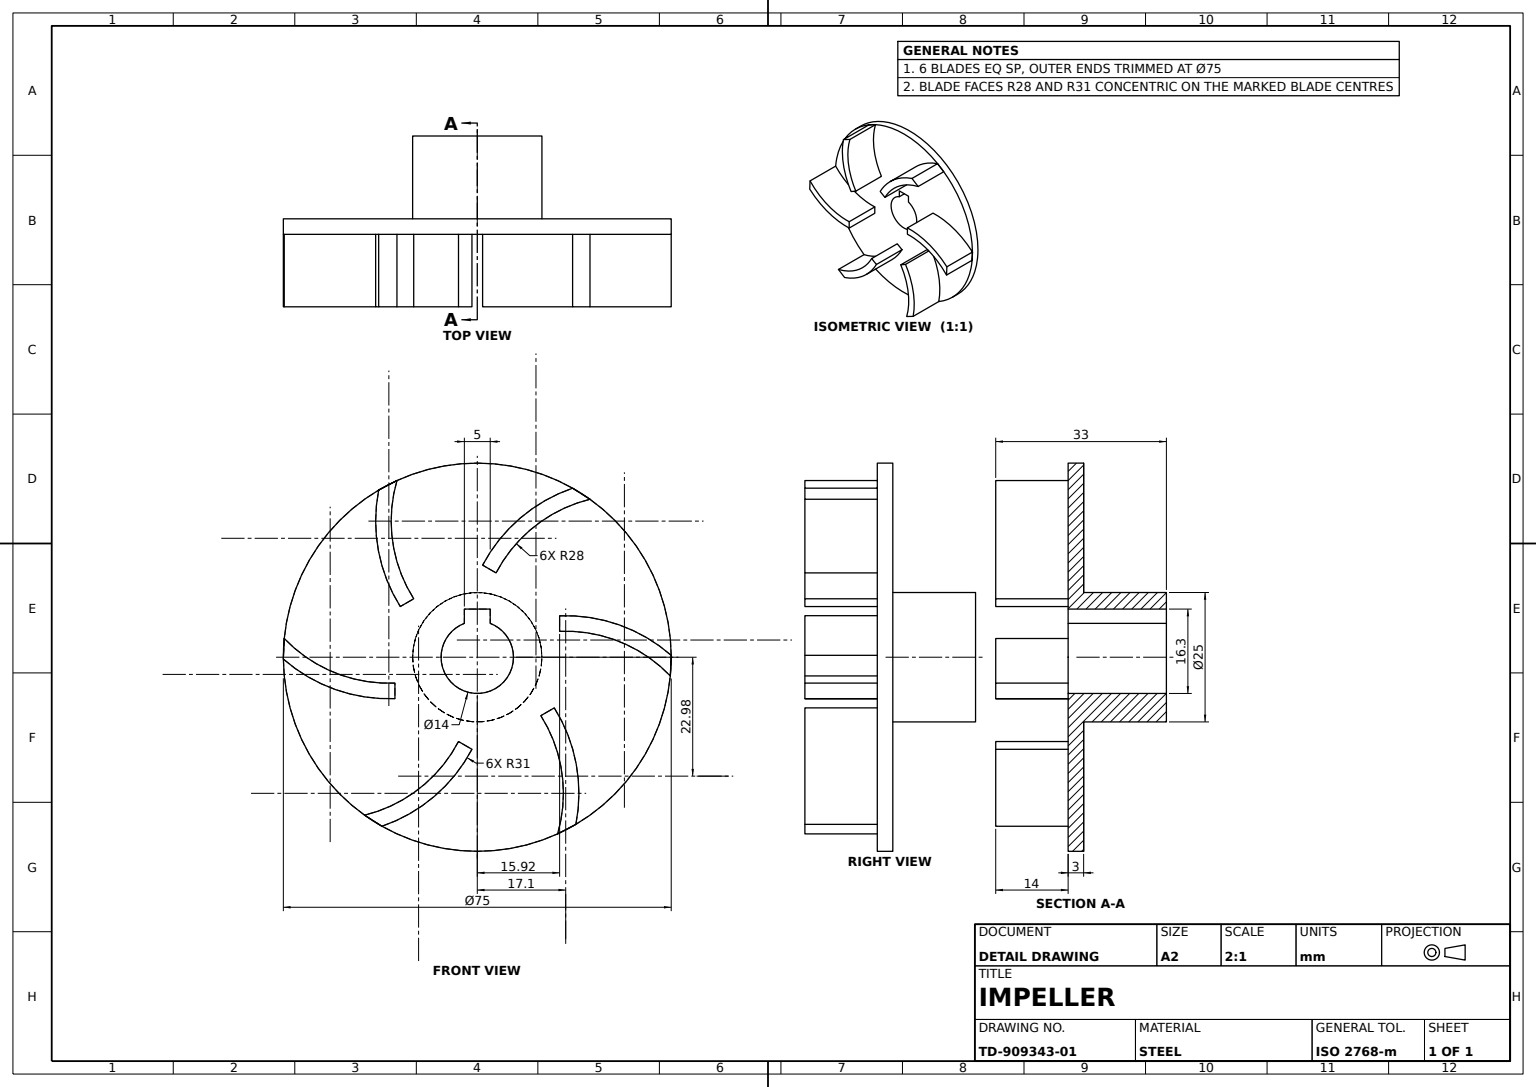
SolidWorks part; units mm, degrees
material "Plain Carbon Steel"
ref_plane "Front Plane" through (0, 0, 0) normal (0, 0, 1) x (1, 0, 0)
ref_plane "Top Plane" through (0, 0, 0) normal (0, 1, 0) x (1, 0, 0)
ref_plane "Right Plane" through (0, 0, 0) normal (1, 0, 0) x (0, 0, -1)
sketch "Back Disc Sketch" plane through (0, 0, 0) normal (0, 0, 1) x (1, 0, 0)
  circle A0 centre (0, 0) radius 37.5
  dimension "D1" = 75
extrude "Back Disc Ø75" add sketch "Back Disc Sketch" along normal blind 3
sketch "Blade Profiles Sketch" plane through (0, 0, 3) normal (0, 0, 1) x (1, 0, 0)
  line L0 (-37.5, 0) -> (37.5, 0) construction
  line L1 (-27.5522, -3) -> (-38.3396, -3) construction
  line L2 (-37.3254, 3.614) -> (-37.4982, -0.3665)
  line L3 (-15.922, -5) -> (-15.922, -8.0024)
  line L4 (-15.5329, 34.1318) -> (-19.0665, 32.2911)
  line L5 (-12.2911, 11.2888) -> (-14.8913, 9.7876)
  line L6 (21.7925, 30.5178) -> (18.4317, 32.6577)
  line L7 (3.6308, 16.2888) -> (1.0307, 17.79)
  line L8 (37.3254, -3.614) -> (37.4982, 0.3665)
  line L9 (15.922, 5) -> (15.922, 8.0024)
  line L10 (15.5329, -34.1318) -> (19.0665, -32.2911)
  line L11 (12.2911, -11.2888) -> (14.8913, -9.7876)
  line L12 (-21.7925, -30.5178) -> (-18.4317, -32.6577)
  line L13 (-3.6308, -16.2888) -> (-1.0307, -17.79)
  circle A0 centre (0, 0) radius 37.5 construction
  arc A1 (-37.3254, 3.614) -> (-15.922, -5) centre (-17.0982, 22.9753) ccw
  arc A2 (-37.4982, -0.3665) -> (-15.7959, -7.9974) centre (-17.0982, 22.9753) ccw
  arc A3 (-15.5329, 34.1318) -> (-12.2911, 11.2888) centre (11.3481, 26.2951) ccw
  arc A4 (-39.4927, 1.5396) -> (-15.7959, -7.9974) centre (-17.0982, 22.9753) ccw construction
  arc A5 (-19.0665, 32.2911) -> (-14.8239, 9.681) centre (11.3481, 26.2951) ccw
  arc A6 (21.7925, 30.5178) -> (3.6308, 16.2888) centre (28.4463, 3.3199) ccw
  arc A7 (18.4317, 32.6577) -> (0.9721, 17.6783) centre (28.4463, 3.3199) ccw
  arc A8 (37.3254, -3.614) -> (15.922, 5) centre (17.0982, -22.9753) ccw
  arc A9 (37.4982, 0.3665) -> (15.7959, 7.9974) centre (17.0982, -22.9753) ccw
  arc A10 (15.5329, -34.1318) -> (12.2911, -11.2888) centre (-11.3481, -26.2951) ccw
  arc A11 (19.0665, -32.2911) -> (14.8239, -9.681) centre (-11.3481, -26.2951) ccw
  arc A12 (-21.7925, -30.5178) -> (-3.6308, -16.2888) centre (-28.4463, -3.3199) ccw
  arc A13 (-18.4317, -32.6577) -> (-0.9721, -17.6783) centre (-28.4463, -3.3199) ccw
  point P53 (0, 0)
  dimension "D1" = 28
  dimension "D3" = 3.0024
  dimension "D4" = 3
  dimension "D5" = 5
  dimension "D2" = 3
  dimension "D6" = 6
extrude "Blades 6x" add sketch "Blade Profiles Sketch" along normal blind 14 contours L6 A7 L7 A6 | L4 A5 L5 A3 | L2 A2 L3 A1 | L12 A13 L13 A12 | L10 A11 L11 A10 | L8 A9 L9 A8
sketch "Hub Sketch" plane through (0, 0, 0) normal (0, 0, -1) x (-1, 0, 0)
  circle A0 centre (0, 0) radius 12.5
  dimension "D1" = 25
extrude "Hub Ø25" add sketch "Hub Sketch" along normal blind 16
sketch "Shaft Bore Sketch" plane through (0, 0, -16) normal (0, 0, -1) x (-1, 0, 0)
  line L0 (0, 24.0084) -> (0, -7) construction
  line L1 (-2.5, 6.5383) -> (-2.5, 9.3)
  line L2 (-2.5, 9.3) -> (2.5, 9.3)
  line L3 (2.5, 9.3) -> (2.5, 6.5383)
  line L4 (0, -7) -> (3.3833, -6.6827) construction
  arc A0 (-2.5, 6.5383) -> (2.5, 6.5383) centre (0, 0) ccw
  dimension "D1" = 14
  dimension "D2" = 5
  dimension "D3" = 16.3
  dimension "D4" = 31.0084
  dimension "D5" = 3.3982
  dimension "D6" = 95.358
extrude "Keyed Shaft Bore Ø14" cut sketch "Shaft Bore Sketch" against normal through all
